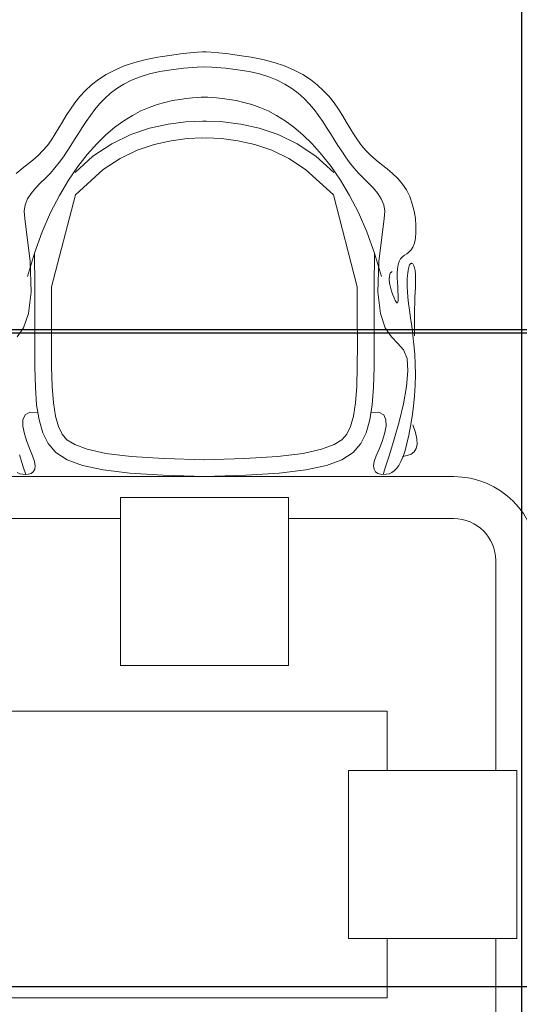
# Model space of a CAD drawing. Units: inches. Extents: x 1454 to 2136, y 626 to 1213.
# Tile 16 of 23: x 1678 to 1701, y 1095 to 1141. Entities that reach past the tile are written whole.
import ezdxf

# ---------------------------------------------------------------- set-up
doc = ezdxf.new("R2010")
doc.units = ezdxf.units.IN
doc.header["$MEASUREMENT"] = 0
for name, color, linetype, lineweight in [('A-ANNO-DIMS', 2, 'Continuous', 18), ('A-FURN-PATT', 252, 'Continuous', 13), ('conference', 41, 'Continuous', 18)]:
    doc.layers.add(name, color=color, linetype=linetype, lineweight=lineweight)
doc.styles.get("Standard").update_dxf_attribs({"font": 'arial.ttf'})
doc.dimstyles.get("Standard").update_dxf_attribs({"dimtxt": 4, "dimasz": 0.18, "dimexe": 0.18, "dimexo": 0.0625, "dimgap": 0.09, "dimtad": 0, "dimtih": 1, "dimtoh": 1, "dimdec": 0, "dimrnd": 6, "dimzin": 0, "dimdsep": 46, "dimlunit": 3, "dimtxsty": 'Standard', "dimcen": 0.09, "dimadec": 0, "dimazin": 0, "dimtfac": 1, "dimtdec": 0, "dimtofl": 0, "dimtmove": 0, "dimatfit": 3, "dimfxl": 1, "dimtolj": 1, "dimtzin": 0, "dimarcsym": 0})

# ---------------------------------------------------------------- blocks, each defined once
blk = doc.blocks.new('ОГ52_на12персон_стол2800х900')
for p, q in [((920.4, 772.5), (933.9, 776)), ((933.9, 776), (948, 778.8)), ((948, 778.8), (961.8, 780.9)), ((961.8, 780.9), (974.8, 782.6)), ((974.8, 782.6), (986.2, 783.7)), ((986.2, 783.7), (995.2, 784.5)), ((995.2, 784.5), (1001.2, 784.9)), ((1001.2, 784.9), (1003.4, 785)), ((1005.6, 784.9), (1003.4, 785)), ((1011.5, 784.5), (1005.6, 784.9)), ((1020.6, 783.7), (1011.5, 784.5)), ((1031.9, 782.6), (1020.6, 783.7)), ((1044.9, 780.9), (1031.9, 782.6)), ((1058.8, 778.8), (1044.9, 780.9)), ((1072.8, 776), (1058.8, 778.8)), ((1086.4, 772.5), (1072.8, 776)), ((886.5, 758), (896.6, 763.4)), ((896.6, 763.4), (907.9, 768.3)), ((907.9, 768.3), (920.4, 772.5)), ((950.1, 761.5), (963.6, 763.8)), ((963.6, 763.8), (978.4, 765.6)), ((978.4, 765.6), (994.8, 766.8)), ((994.8, 766.8), (1003.4, 767.1)), ((1012, 766.8), (1003.4, 767.1)), ((1028.3, 765.6), (1012, 766.8)), ((1043.1, 763.8), (1028.3, 765.6)), ((1056.7, 761.5), (1043.1, 763.8)), ((1098.8, 768.3), (1086.4, 772.5)), ((1110.1, 763.4), (1098.8, 768.3)), ((1120.3, 758), (1110.1, 763.4)), ((869, 745.6), (877.3, 752)), ((877.3, 752), (886.5, 758)), ((907.5, 746.6), (916.6, 751.2)), ((916.6, 751.2), (926.7, 755.2)), ((926.7, 755.2), (937.8, 758.7)), ((937.8, 758.7), (950.1, 761.5)), ((1068.9, 758.7), (1056.7, 761.5)), ((1080, 755.2), (1068.9, 758.7)), ((1090.1, 751.2), (1080, 755.2)), ((1099.2, 746.6), (1090.1, 751.2)), ((1129.5, 752), (1120.3, 758)), ((1137.7, 745.6), (1129.5, 752)), ((855, 731.7), (861.6, 738.8)), ((861.6, 738.8), (869, 745.6)), ((891.7, 735.7), (899.2, 741.4)), ((899.2, 741.4), (907.5, 746.6)), ((1107.5, 741.4), (1099.2, 746.6)), ((1115, 735.7), (1107.5, 741.4)), ((1145.1, 738.8), (1137.7, 745.6)), ((1151.7, 731.7), (1145.1, 738.8)), ((849.1, 724.4), (855, 731.7)), ((878.6, 723.1), (884.9, 729.6)), ((884.9, 729.6), (891.7, 735.7)), ((956.3, 724.9), (965.4, 727)), ((965.4, 727), (974.1, 728.5)), ((974.1, 728.5), (982, 729.6)), ((982, 729.6), (989.1, 730.4)), ((989.1, 730.4), (994.9, 730.8)), ((994.9, 730.8), (999.4, 731)), ((999.4, 731), (1002.3, 731.1)), ((1002.3, 731.1), (1003.4, 731.1)), ((1004.4, 731.1), (1003.4, 731.1)), ((1007.3, 731), (1004.4, 731.1)), ((1011.8, 730.8), (1007.3, 731)), ((1017.7, 730.4), (1011.8, 730.8)), ((1024.7, 729.6), (1017.7, 730.4)), ((1032.7, 728.5), (1024.7, 729.6)), ((1041.3, 727), (1032.7, 728.5)), ((1050.4, 724.9), (1041.3, 727)), ((1121.9, 729.6), (1115, 735.7)), ((1128.1, 723.1), (1121.9, 729.6)), ((1157.6, 724.4), (1151.7, 731.7)), ((839, 709.4), (843.8, 716.9)), ((843.8, 716.9), (849.1, 724.4)), ((867.6, 709.3), (872.9, 716.3)), ((872.9, 716.3), (878.6, 723.1)), ((927.6, 714.7), (937.4, 718.9)), ((937.4, 718.9), (947, 722.3)), ((947, 722.3), (956.3, 724.9)), ((1059.7, 722.3), (1050.4, 724.9)), ((1069.3, 718.9), (1059.7, 722.3)), ((1079.1, 714.7), (1069.3, 718.9)), ((1133.9, 716.3), (1128.1, 723.1)), ((1139.2, 709.3), (1133.9, 716.3)), ((1162.9, 716.9), (1157.6, 724.4)), ((1167.7, 709.4), (1162.9, 716.9)), ((834.5, 701.9), (839, 709.4)), ((862.6, 702.2), (867.6, 709.3)), ((907.4, 703), (917.6, 709.4)), ((917.6, 709.4), (927.6, 714.7)), ((1089.1, 709.4), (1079.1, 714.7)), ((1099.4, 703), (1089.1, 709.4)), ((1144.1, 702.2), (1139.2, 709.3)), ((1172.2, 701.9), (1167.7, 709.4)), ((825.8, 687.3), (830.2, 694.5)), ((830.2, 694.5), (834.5, 701.9)), ((853.4, 687.9), (857.9, 695)), ((857.9, 695), (862.6, 702.2)), ((886.2, 686.1), (896.9, 695.3)), ((896.9, 695.3), (907.4, 703)), ((915.6, 686.5), (938.1, 694.2)), ((938.1, 694.2), (960.2, 699)), ((960.2, 699), (981.3, 701.6)), ((981.3, 701.6), (1001, 702.5)), ((1001, 702.5), (1003.4, 702.4)), ((1005.7, 702.5), (1003.4, 702.4)), ((1025.4, 701.6), (1005.7, 702.5)), ((1046.5, 699), (1025.4, 701.6)), ((1068.6, 694.2), (1046.5, 699)), ((1091.2, 686.5), (1068.6, 694.2)), ((1109.9, 695.3), (1099.4, 703)), ((1120.6, 686.1), (1109.9, 695.3)), ((1148.8, 695), (1144.1, 702.2)), ((1153.4, 687.9), (1148.8, 695)), ((1176.6, 694.5), (1172.2, 701.9)), ((1180.9, 687.3), (1176.6, 694.5)), ((816.5, 673.7), (821.3, 680.3)), ((821.3, 680.3), (825.8, 687.3)), ((844.5, 673.7), (848.9, 680.7)), ((848.9, 680.7), (853.4, 687.9)), ((875.2, 675.4), (886.2, 686.1)), ((893, 675.6), (915.6, 686.5)), ((963.6, 679.3), (983, 681.7)), ((983, 681.7), (1001.3, 682.5)), ((1001.3, 682.5), (1003, 682.4)), ((1005.5, 682.5), (1003.8, 682.4)), ((1023.8, 681.7), (1005.5, 682.5)), ((1043.1, 679.3), (1023.8, 681.7)), ((1113.8, 675.6), (1091.2, 686.5)), ((1131.5, 675.4), (1120.6, 686.1)), ((1157.8, 680.7), (1153.4, 687.9)), ((1162.2, 673.7), (1157.8, 680.7)), ((1185.4, 680.3), (1180.9, 687.3)), ((1190.3, 673.7), (1185.4, 680.3)), ((811.2, 667.5), (816.5, 673.7)), ((840.1, 666.7), (844.5, 673.7)), ((864, 663), (875.2, 675.4)), ((870.7, 660.8), (893, 675.6)), ((923.2, 668), (943.5, 674.9)), ((943.5, 674.9), (963.6, 679.3)), ((1063.2, 674.9), (1043.1, 679.3)), ((1083.6, 668), (1063.2, 674.9)), ((1136, 660.8), (1113.8, 675.6)), ((1142.7, 663), (1131.5, 675.4)), ((1166.7, 666.7), (1162.2, 673.7)), ((1195.6, 667.5), (1190.3, 673.7)), ((799, 656.2), (805.3, 661.7)), ((805.3, 661.7), (811.2, 667.5)), ((830.6, 653.3), (835.5, 659.9)), ((835.5, 659.9), (840.1, 666.7)), ((849.4, 641.6), (870.7, 660.8)), ((852.8, 648.7), (864, 663)), ((883, 644.9), (902.9, 658.2)), ((902.9, 658.2), (923.2, 668)), ((1103.8, 658.2), (1083.6, 668)), ((1123.7, 644.9), (1103.8, 658.2)), ((1157.3, 641.6), (1136, 660.8)), ((1154, 648.7), (1142.7, 663)), ((1171.3, 659.9), (1166.7, 666.7)), ((1176.1, 653.3), (1171.3, 659.9)), ((1201.4, 661.7), (1195.6, 667.5)), ((1207.7, 656.2), (1201.4, 661.7)), ((779.5, 640.1), (785.9, 645.6)), ((785.9, 645.6), (792.5, 650.9)), ((792.5, 650.9), (799, 656.2)), ((820, 640.6), (825.5, 646.8)), ((825.5, 646.8), (830.6, 653.3)), ((841.6, 632.4), (852.8, 648.7)), ((849.8, 615), (883, 644.9)), ((1157, 615), (1123.7, 644.9)), ((1165.2, 632.4), (1154, 648.7)), ((1181.3, 646.8), (1176.1, 653.3)), ((1186.8, 640.6), (1181.3, 646.8)), ((1214.2, 650.9), (1207.7, 656.2)), ((1220.8, 645.6), (1214.2, 650.9)), ((1227.3, 640.1), (1220.8, 645.6)), ((808, 628.7), (814.1, 634.6)), ((814.1, 634.6), (820, 640.6)), ((1192.7, 634.6), (1186.8, 640.6)), ((1198.7, 628.7), (1192.7, 634.6)), ((1233.4, 634.2), (1227.3, 640.1)), ((1238.9, 627.7), (1233.4, 634.2)), ((797.1, 616.6), (802.3, 622.8)), ((802.3, 622.8), (808, 628.7)), ((830.7, 614.1), (841.6, 632.4)), ((1176.1, 614.1), (1165.2, 632.4)), ((1204.5, 622.8), (1198.7, 628.7)), ((1209.6, 616.6), (1204.5, 622.8)), ((1243.7, 620.6), (1238.9, 627.7)), ((790, 603), (792.9, 610.1)), ((792.9, 610.1), (797.1, 616.6)), ((820.1, 593.6), (830.7, 614.1)), ((849.8, 615), (821.5, 505.2)), ((1157, 615), (1185.3, 505.2)), ((1186.6, 593.6), (1176.1, 614.1)), ((1213.8, 610.1), (1209.6, 616.6)), ((1216.7, 603), (1213.8, 610.1)), ((1247.7, 612.7), (1243.7, 620.6)), ((1250.7, 604.2), (1247.7, 612.7)), ((788.8, 595.2), (790, 603)), ((1217.9, 595.2), (1216.7, 603)), ((1253, 595.4), (1250.7, 604.2)), ((789.6, 586.5), (788.8, 595.2)), ((789.6, 586.5), (796, 535.5)), ((810.2, 570.7), (820.1, 593.6)), ((1196.5, 570.7), (1186.6, 593.6)), ((1217.1, 586.5), (1210.8, 535.5)), ((1217.1, 586.5), (1217.9, 595.2)), ((1254.4, 586.6), (1253, 595.4)), ((1255.1, 578.1), (1254.4, 586.6)), ((1255.1, 570.2), (1255.1, 578.1)), ((801, 545.4), (810.2, 570.7)), ((1205.7, 545.4), (1196.5, 570.7)), ((1253.2, 557.2), (1254.5, 563.1)), ((1254.5, 563.1), (1255.1, 570.2)), ((1249.2, 549.3), (1251.4, 552.7)), ((1251.4, 552.7), (1253.2, 557.2)), ((792.7, 517.6), (801, 545.4)), ((801, 545.4), (801.5, 505.1)), ((1205.7, 545.4), (1205.3, 505.1)), ((1214, 517.6), (1205.7, 545.4)), ((1236.9, 538.5), (1239.1, 540.8)), ((1239.1, 540.8), (1241.5, 542.8)), ((1241.5, 542.8), (1244.1, 544.6)), ((1244.1, 544.6), (1246.7, 546.7)), ((1246.7, 546.7), (1249.2, 549.3)), ((796, 535.5), (797, 498.8)), ((1210.8, 535.5), (1209.7, 498.8)), ((1233.3, 526.8), (1234, 531.5)), ((1234, 531.5), (1235.2, 535.5)), ((1235.2, 535.5), (1236.9, 538.5)), ((1246.2, 527), (1246.6, 528.8)), ((1246.6, 528.8), (1247.1, 530.3)), ((1247.1, 530.3), (1247.6, 531.5)), ((1247.6, 531.5), (1248.1, 532.3)), ((1248.1, 532.3), (1248.7, 532.9)), ((1248.7, 532.9), (1249.2, 533.2)), ((1249.2, 533.2), (1249.7, 533.3)), ((1249.7, 533.3), (1250.2, 533.2)), ((1250.2, 533.2), (1250.7, 533)), ((1250.7, 533), (1251.2, 532.5)), ((1251.2, 532.5), (1251.6, 531.9)), ((1251.6, 531.9), (1252.1, 531.1)), ((1252.1, 531.1), (1252.5, 530.2)), ((1252.5, 530.2), (1252.9, 529.1)), ((1252.9, 529.1), (1253.3, 527.9)), ((1253.3, 527.9), (1253.6, 526.5)), ((1223.5, 518.2), (1223.3, 514.2)), ((1224.6, 521.4), (1223.5, 518.2)), ((1226.8, 523.4), (1224.6, 521.4)), ((1232.9, 521.5), (1233.3, 526.8)), ((1232.9, 516), (1232.9, 521.5)), ((1233.1, 510.3), (1232.9, 516)), ((1244.8, 514.9), (1245, 518.7)), ((1245, 518.7), (1245.3, 521.9)), ((1245.3, 521.9), (1245.7, 524.7)), ((1245.7, 524.7), (1246.2, 527)), ((1253.6, 526.5), (1254, 524.9)), ((1254, 524.9), (1254.2, 523.1)), ((1254.2, 523.1), (1254.5, 521)), ((1254.5, 521), (1254.6, 518.5)), ((1254.6, 518.5), (1254.7, 515.7)), ((801.5, 505.1), (801.5, 469.2)), ((821.5, 505.2), (821.5, 469.2)), ((1185.3, 505.2), (1185.3, 469.2)), ((1205.3, 505.1), (1205.3, 469.2)), ((1223.3, 514.2), (1223.7, 509.6)), ((1223.7, 509.6), (1224.7, 504.8)), ((1224.7, 504.8), (1226.1, 500.1)), ((1233.4, 504.9), (1233.1, 510.3)), ((1233.7, 499.8), (1233.4, 504.9)), ((1244.7, 510.5), (1244.8, 514.9)), ((1244.8, 505.4), (1244.7, 510.5)), ((1245.1, 499.6), (1244.8, 505.4)), ((1254.6, 508.5), (1254.5, 504)), ((1254.7, 512.3), (1254.6, 508.5)), ((1254.7, 515.7), (1254.7, 512.3)), ((797, 498.8), (794, 473.4)), ((1209.7, 498.8), (1212.8, 473.4)), ((1226.1, 500.1), (1227.6, 495.7)), ((1227.6, 495.7), (1229, 492)), ((1233.9, 495.4), (1233.7, 499.8)), ((1233.9, 491.8), (1233.9, 495.4)), ((1245.6, 493.1), (1245.1, 499.6)), ((1246.4, 485.6), (1245.6, 493.1)), ((1253.9, 493), (1253.7, 486.1)), ((1254.2, 498.9), (1253.9, 493)), ((1254.5, 504), (1254.2, 498.9)), ((1229, 492), (1230.3, 489.2)), ((1230.3, 489.2), (1231.4, 487.3)), ((1231.4, 487.3), (1232.3, 486.4)), ((1232.3, 486.4), (1233, 486.4)), ((1233, 486.4), (1233.5, 487.3)), ((1233.5, 487.3), (1233.8, 489.1)), ((1233.8, 489.1), (1233.9, 491.8)), ((1247.4, 477.3), (1246.4, 485.6)), ((1253.7, 486.1), (1253.4, 478.2)), ((794, 473.4), (788.1, 456.6)), ((801.5, 469.2), (801.4, 437.5)), ((821.5, 469.2), (821.4, 437.6)), ((1185.3, 469.2), (1185.4, 437.6)), ((1205.3, 469.2), (1205.4, 437.5)), ((1212.8, 473.4), (1218.6, 456.6)), ((1248.7, 468.2), (1247.4, 477.3)), ((1253.4, 478.2), (1253.3, 469.2)), ((1253.3, 469.2), (1253.3, 458.8)), ((1250, 458.3), (1248.7, 468.2)), ((1251.4, 447.8), (1250, 458.3)), ((1253.3, 458.8), (1253.4, 447.1)), ((788.1, 456.6), (780.7, 445.7)), ((1218.6, 456.6), (1226, 445.7)), ((1226, 445.7), (1233.6, 437.8)), ((1252.6, 436.7), (1251.4, 447.8)), ((801.4, 437.5), (801.5, 409.8)), ((821.4, 437.6), (821.5, 410.1)), ((1185.4, 437.6), (1185.3, 410.1)), ((1205.4, 437.5), (1205.3, 409.8)), ((1233.6, 437.8), (1240.2, 430.2)), ((1253.6, 425.1), (1252.6, 436.7)), ((1240.2, 430.2), (1244.5, 420)), ((1254.2, 413.1), (1253.6, 425.1)), ((1244.5, 420), (1245.6, 405.3)), ((1254.4, 400.7), (1254.2, 413.1)), ((801.5, 409.8), (802.2, 385.6)), ((821.5, 410.1), (822.1, 386.6)), ((1185.3, 410.1), (1184.6, 386.6)), ((1205.3, 409.8), (1204.6, 385.6)), ((1245.6, 405.3), (1243.9, 386.7)), ((1254.1, 388.2), (1254.4, 400.7)), ((1253.4, 375.5), (1254.1, 388.2)), ((802.2, 385.6), (803.7, 364.7)), ((822.1, 386.6), (823.6, 367)), ((1184.6, 386.6), (1183.1, 367)), ((1204.6, 385.6), (1203, 364.7)), ((1243.9, 386.7), (1240.1, 366)), ((1252.1, 363), (1253.4, 375.5)), ((803.7, 364.7), (806.5, 346.8)), ((823.6, 367), (826.1, 351.1)), ((1183.1, 367), (1180.6, 351.1)), ((1203, 364.7), (1200.2, 346.8)), ((1240.1, 366), (1235, 344.5)), ((787.3, 347.1), (789.9, 353)), ((789.9, 353), (795.6, 356.1)), ((795.6, 356.1), (805.1, 355.7)), ((1211.1, 356.1), (1201.6, 355.7)), ((1216.8, 353), (1211.1, 356.1)), ((1219.4, 347.1), (1216.8, 353)), ((1250.6, 350.9), (1252.1, 363)), ((787.3, 339.3), (787.3, 347.1)), ((806.5, 346.8), (810.9, 331.5)), ((826.1, 351.1), (829.6, 338.8)), ((1180.6, 351.1), (1177.1, 338.8)), ((1200.2, 346.8), (1195.9, 331.5)), ((1219.5, 339.3), (1219.4, 347.1)), ((1235, 344.5), (1229.2, 323.8)), ((1248.7, 339.4), (1250.6, 350.9)), ((1251.4, 341), (1254.7, 331.8)), ((789.1, 330.3), (787.3, 339.3)), ((792, 321), (789.1, 330.3)), ((810.9, 331.5), (817.3, 318.7)), ((829.6, 338.8), (834, 329.9)), ((834, 329.9), (839.8, 323.3)), ((1172.7, 329.9), (1166.9, 323.3)), ((1177.1, 338.8), (1172.7, 329.9)), ((1195.9, 331.5), (1189.5, 318.7)), ((1214.7, 321), (1217.7, 330.3)), ((1217.7, 330.3), (1219.5, 339.3)), ((1244.4, 318.9), (1246.6, 328.7)), ((1246.6, 328.7), (1248.7, 339.4)), ((1254.7, 331.8), (1256.3, 324.1)), ((795.5, 312), (792, 321)), ((817.3, 318.7), (826.6, 308)), ((839.8, 323.3), (849, 317.4)), ((849, 317.4), (863.9, 311.8)), ((1157.8, 317.4), (1142.8, 311.8)), ((1166.9, 323.3), (1157.8, 317.4)), ((1189.5, 318.7), (1180.2, 308)), ((1211.2, 312), (1214.7, 321)), ((1229.2, 323.8), (1223.6, 305.4)), ((1242.1, 310.4), (1244.4, 318.9)), ((1256.5, 317.8), (1255.3, 312.9)), ((1256.3, 324.1), (1256.5, 317.8)), ((783.1, 305.4), (787.8, 291)), ((798.9, 304.2), (795.5, 312)), ((826.6, 308), (839.9, 299.4)), ((863.9, 311.8), (886.1, 307)), ((886.1, 307), (916.3, 303.4)), ((1120.7, 307), (1090.5, 303.4)), ((1142.8, 311.8), (1120.7, 307)), ((1180.2, 308), (1166.8, 299.4)), ((1207.8, 304.2), (1211.2, 312)), ((1223.6, 305.4), (1218.9, 291)), ((1239.7, 303.2), (1242.1, 310.4)), ((1249.2, 306.2), (1244.6, 304.3)), ((1252.8, 309), (1249.2, 306.2)), ((1255.3, 312.9), (1252.8, 309)), ((798.9, 304.2), (801.3, 297.4)), ((801.3, 297.4), (802.1, 292.1)), ((839.9, 299.4), (858.3, 292.5)), ((916.3, 303.4), (955.2, 300.9)), ((955.2, 300.9), (1004, 299.3)), ((1051.5, 300.9), (1002.7, 299.3)), ((1090.5, 303.4), (1051.5, 300.9)), ((1166.8, 299.4), (1148.5, 292.5)), ((1205.4, 297.4), (1204.6, 292.1)), ((1207.8, 304.2), (1205.4, 297.4)), ((1234.7, 292.5), (1237.2, 297.3)), ((1237.2, 297.3), (1239.7, 303.2)), ((1244.6, 304.3), (1239.1, 303.1)), ((783.6, 282.8), (780.4, 284.1)), ((786.9, 282.1), (783.6, 282.8)), ((790.4, 281.8), (786.9, 282.1)), ((787.8, 291), (790.9, 281.9)), ((793.9, 282.2), (790.4, 281.8)), ((797.1, 283.2), (793.9, 282.2)), ((799.7, 285.1), (797.1, 283.2)), ((801.5, 288.1), (799.7, 285.1)), ((802.1, 292.1), (801.5, 288.1)), ((858.3, 292.5), (882.8, 287.3)), ((882.8, 287.3), (914.4, 283.5)), ((914.4, 283.5), (954.3, 280.9)), ((1092.3, 283.5), (1052.5, 280.9)), ((1124, 287.3), (1092.3, 283.5)), ((1148.5, 292.5), (1124, 287.3)), ((1204.6, 292.1), (1205.3, 288.1)), ((1205.3, 288.1), (1207, 285.1)), ((1207, 285.1), (1209.6, 283.2)), ((1209.6, 283.2), (1212.8, 282.2)), ((1212.8, 282.2), (1216.3, 281.8)), ((1218.9, 291), (1215.9, 281.9)), ((1216.3, 281.8), (1219.8, 282.1)), ((1219.8, 282.1), (1223.2, 282.8)), ((1223.2, 282.8), (1226.3, 284.1)), ((1226.3, 284.1), (1229.2, 286.1)), ((1229.2, 286.1), (1232, 288.8)), ((1232, 288.8), (1234.7, 292.5)), ((-1300, 279.3), (1300, 279.3)), ((954.3, 280.9), (1003.4, 279.3)), ((1052.5, 280.9), (1003.4, 279.3)), ((903.4, 254.3), (903.4, 54.3)), ((1103.4, 254.3), (903.4, 254.3)), ((1103.4, 54.3), (1103.4, 254.3)), ((603.4, 229.3), (903.4, 229.3)), ((1103.4, 229.3), (1300, 229.3)), ((1350, 179.3), (1350, -70.7)), ((903.4, 54.3), (1103.4, 54.3)), ((1220.7, 0), (-1220.7, 0)), ((1220.7, -70.7), (1220.7, 0)), ((1175, -270.7), (1175, -70.7)), ((1175, -70.7), (1375, -70.7)), ((1375, -70.7), (1375, -270.7)), ((1375, -270.7), (1175, -270.7)), ((1220.7, -341.4), (1220.7, -270.7)), ((1350, -270.7), (1350, -520.7)), ((-1220.7, -341.4), (1220.7, -341.4))]:
    blk.add_line(p, q)
for radius in [100, 50]:
    blk.add_arc((1300, 179.3), radius, 0, 90)
blk = doc.blocks.new('*D23')
at = {"layer": 'A-ANNO-DIMS', "color": 0, "lineweight": -2, "transparency": 16777216}
for p, q in [((1571.674, 1139.532), (1571.674, 1162.157)), ((1571.854, 1161.977), (1615.675, 1161.977)), ((1721.545, 1161.977), (1677.724, 1161.977)), ((1721.725, 1139.532), (1721.725, 1162.157))]:
    blk.add_line(p, q, dxfattribs=at)
at = {"layer": 'A-ANNO-DIMS', "color": 0, "transparency": 16777216}
for points in [[(1571.854, 1162.007), (1571.854, 1161.947), (1571.674, 1161.977)], [(1721.545, 1162.007), (1721.545, 1161.947), (1721.725, 1161.977)]]:
    blk.add_solid(points, dxfattribs=at)
at = {"layer": 'Defpoints', "color": 0, "transparency": 16777216}
for p in [(1721.725, 1161.977), (1571.674, 1139.469), (1721.725, 1139.469)]:
    blk.add_point(p, dxfattribs=at)
at = {"layer": 'A-ANNO-DIMS', "color": 0, "transparency": 16777216, "insert": (1646.7, 1161.977), "char_height": 4, "attachment_point": 5}
blk.add_mtext('\\A1;CONFERENCE SET 150', dxfattribs=at)
blk = doc.blocks.new('*D33')
at = {"layer": 'A-ANNO-DIMS', "color": 0, "lineweight": -2, "transparency": 16777216}
for p, q in [((2032.494, 1126.282), (1462.374, 1126.282)), ((1462.554, 1126.102), (1462.554, 1056.381)), ((1462.554, 982.462), (1462.554, 1052.184)), ((2032.494, 982.282), (1462.374, 982.282))]:
    blk.add_line(p, q, dxfattribs=at)
at = {"layer": 'A-ANNO-DIMS', "color": 0, "transparency": 16777216}
for points in [[(1462.524, 1126.102), (1462.584, 1126.102), (1462.554, 1126.282)], [(1462.524, 982.462), (1462.584, 982.462), (1462.554, 982.282)]]:
    blk.add_solid(points, dxfattribs=at)
at = {"layer": 'Defpoints', "color": 0, "transparency": 16777216}
for p in [(1462.554, 1126.282), (2032.556, 1126.282), (2032.556, 982.282)]:
    blk.add_point(p, dxfattribs=at)
at = {"layer": 'A-ANNO-DIMS', "color": 0, "transparency": 16777216, "insert": (1462.554, 1054.282), "char_height": 4, "attachment_point": 5}
blk.add_mtext('\\A1;144', dxfattribs=at)
blk = doc.blocks.new('*D45')
at = {"layer": 'A-ANNO-DIMS', "color": 0, "lineweight": -2, "transparency": 16777216}
for p, q in [((1654.556, 913.345), (1654.556, 1210.464)), ((1654.736, 1210.284), (1670.917, 1210.284)), ((1700.896, 1210.284), (1684.715, 1210.284)), ((1701.076, 909.11), (1701.076, 1210.464))]:
    blk.add_line(p, q, dxfattribs=at)
at = {"layer": 'A-ANNO-DIMS', "color": 0, "transparency": 16777216}
for points in [[(1654.736, 1210.314), (1654.736, 1210.254), (1654.556, 1210.284)], [(1700.896, 1210.314), (1700.896, 1210.254), (1701.076, 1210.284)]]:
    blk.add_solid(points, dxfattribs=at)
at = {"layer": 'Defpoints', "color": 0, "transparency": 16777216}
for p in [(1701.076, 1210.284), (1654.556, 913.282), (1701.076, 909.048)]:
    blk.add_point(p, dxfattribs=at)
at = {"layer": 'A-ANNO-DIMS', "color": 0, "transparency": 16777216, "insert": (1677.816, 1210.284), "char_height": 4, "attachment_point": 5}
blk.add_mtext('\\A1;46.52', dxfattribs=at)
blk = doc.blocks.new('*D54')
at = {"layer": 'A-ANNO-DIMS', "color": 0, "lineweight": -2, "transparency": 16777216}
for p, q in [((1879.494, 1126.282), (1462.374, 1126.282)), ((1462.554, 1126.102), (1462.554, 1078.915)), ((1462.554, 1027.462), (1462.554, 1074.65)), ((1879.494, 1027.282), (1462.374, 1027.282))]:
    blk.add_line(p, q, dxfattribs=at)
at = {"layer": 'A-ANNO-DIMS', "color": 0, "transparency": 16777216}
for points in [[(1462.524, 1126.102), (1462.584, 1126.102), (1462.554, 1126.282)], [(1462.524, 1027.462), (1462.584, 1027.462), (1462.554, 1027.282)]]:
    blk.add_solid(points, dxfattribs=at)
at = {"layer": 'Defpoints', "color": 0, "transparency": 16777216}
for p in [(1879.556, 1126.282), (1462.554, 1027.282), (1879.556, 1027.282)]:
    blk.add_point(p, dxfattribs=at)
at = {"layer": 'A-ANNO-DIMS', "color": 0, "transparency": 16777216, "insert": (1462.554, 1076.782), "char_height": 4, "attachment_point": 5}
blk.add_mtext('\\A1;99', dxfattribs=at)
blk = doc.blocks.new('*D68')
at = {"layer": 'A-ANNO-DIMS', "color": 0, "lineweight": -2, "transparency": 16777216}
for p, q in [((1659.724, 1027.329), (1659.724, 1210.464)), ((1659.904, 1210.284), (1675.092, 1210.284)), ((1704.128, 1210.284), (1688.939, 1210.284)), ((1704.308, 1027.329), (1704.308, 1210.464))]:
    blk.add_line(p, q, dxfattribs=at)
at = {"layer": 'A-ANNO-DIMS', "color": 0, "transparency": 16777216}
for points in [[(1659.904, 1210.314), (1659.904, 1210.254), (1659.724, 1210.284)], [(1704.128, 1210.314), (1704.128, 1210.254), (1704.308, 1210.284)]]:
    blk.add_solid(points, dxfattribs=at)
at = {"layer": 'Defpoints', "color": 0, "transparency": 16777216}
for p in [(1704.308, 1210.284), (1659.724, 1027.267), (1704.308, 1027.267)]:
    blk.add_point(p, dxfattribs=at)
at = {"layer": 'A-ANNO-DIMS', "color": 0, "transparency": 16777216, "insert": (1682.016, 1210.284), "char_height": 4, "attachment_point": 5}
blk.add_mtext('\\A1;44.58', dxfattribs=at)
blk = doc.blocks.new('*D73')
at = {"layer": 'A-ANNO-DIMS', "color": 0, "lineweight": -2, "transparency": 16777216}
for p, q in [((1985.096, 1126.439), (1462.374, 1126.439)), ((1462.554, 1126.259), (1462.554, 1113.178)), ((1462.554, 1095.83), (1462.554, 1108.911)), ((1966.644, 1095.65), (1462.374, 1095.65))]:
    blk.add_line(p, q, dxfattribs=at)
at = {"layer": 'A-ANNO-DIMS', "color": 0, "transparency": 16777216}
for points in [[(1462.524, 1126.259), (1462.584, 1126.259), (1462.554, 1126.439)], [(1462.524, 1095.83), (1462.584, 1095.83), (1462.554, 1095.65)]]:
    blk.add_solid(points, dxfattribs=at)
at = {"layer": 'Defpoints', "color": 0, "transparency": 16777216}
for p in [(1985.158, 1126.439), (1462.554, 1095.65), (1966.707, 1095.65)]:
    blk.add_point(p, dxfattribs=at)
at = {"layer": 'A-ANNO-DIMS', "color": 0, "transparency": 16777216, "insert": (1462.554, 1111.044), "char_height": 4, "attachment_point": 5}
blk.add_mtext('\\A1;30.79', dxfattribs=at)
blk = doc.blocks.new('*D76')
at = {"layer": 'A-ANNO-DIMS', "color": 0, "lineweight": -2, "transparency": 16777216}
for p, q in [((1962.644, 1095.65), (1462.374, 1095.65)), ((1462.554, 1095.47), (1462.554, 1073.782)), ((1462.554, 1047.83), (1462.554, 1069.517)), ((1914.644, 1047.65), (1462.374, 1047.65))]:
    blk.add_line(p, q, dxfattribs=at)
at = {"layer": 'A-ANNO-DIMS', "color": 0, "transparency": 16777216}
for points in [[(1462.524, 1095.47), (1462.584, 1095.47), (1462.554, 1095.65)], [(1462.524, 1047.83), (1462.584, 1047.83), (1462.554, 1047.65)]]:
    blk.add_solid(points, dxfattribs=at)
at = {"layer": 'Defpoints', "color": 0, "transparency": 16777216}
for p in [(1962.707, 1095.65), (1462.554, 1047.65), (1914.707, 1047.65)]:
    blk.add_point(p, dxfattribs=at)
at = {"layer": 'A-ANNO-DIMS', "color": 0, "transparency": 16777216, "insert": (1462.554, 1071.65), "char_height": 4, "attachment_point": 5}
blk.add_mtext('\\A1;48', dxfattribs=at)

msp = doc.modelspace()

# ---------------------------------------------------------------- hatches: boundary and pattern name
at = {"layer": 'A-FURN-PATT'}
h = msp.add_hatch(dxfattribs=at)
h.set_pattern_fill('ESCHER', color=256)
h.paths.add_polyline_path([(1511.3761, 923.7174, 1), (1525.379, 923.7174, 1)])
h.paths.add_polyline_path([(1525.379, 816.0542, 1), (1511.3761, 816.0542, 1)])
h.paths.add_polyline_path([(1525.379, 712.7345, 1), (1511.3761, 712.7345, 1)])
h.paths.add_polyline_path([(2070.5057, 794.3402, 1), (2056.5027, 794.3402, 1)])
h.paths.add_polyline_path([(2005.868, 1014.5578, 1), (1991.8651, 1014.5578, 1)])
h.paths.add_polyline_path([(1994.0647, 1066.7584, 1), (2008.0677, 1066.7584, 1)])
h.paths.add_polyline_path([(1919.5492, 1065.3848, 1), (1933.5521, 1065.3848, 1)])
h.paths.add_polyline_path([(1936.8517, 1013.7336, 1), (1922.8488, 1013.7336, 1)])
h.paths.add_polyline_path([(1824.6062, 1109.1557, 1), (1838.6091, 1109.1557, 1)])

# ---------------------------------------------------------------- block references
at = {"layer": 'conference', "xscale": 0.0393700787401575, "yscale": 0.0393700787401575, "zscale": 0.0393700787401575}
msp.add_blockref('ОГ52_на12персон_стол2800х900', (1646.6996, 1108.5647), dxfattribs=at)

# ---------------------------------------------------------------- dimensions: what is measured, and where the dimension line sits
at = {"layer": 'A-ANNO-DIMS'}
for base, p1, p2, picture, middle in [((1701.0763, 1210.2845), (1654.5563, 913.2825), (1701.0763, 909.0476), '*D45', (1677.8163, 1210.2845)), ((1704.308, 1210.2845), (1659.7237, 1027.2667), (1704.308, 1027.2667), '*D68', (1682.0158, 1210.2845))]:
    dim = msp.add_linear_dim(base=base, p1=p1, p2=p2, dimstyle='Standard', override={"dimdec": 2, "dimlfac": 1, "dimrnd": 0, "dimzin": 0, "dimdsep": 46, "dimlunit": 2}, dxfattribs=at)
    dim.commit()
    dim.dimension.update_dxf_attribs({"geometry": picture, "text_midpoint": middle})
dim = msp.add_linear_dim(base=(1721.7253, 1161.9768), p1=(1571.674, 1139.4691), p2=(1721.7253, 1139.4691), text='CONFERENCE SET <>', dimstyle='Standard', override={"dimdec": 0, "dimlfac": 1, "dimrnd": 0, "dimzin": 0, "dimdsep": 46, "dimlunit": 2}, dxfattribs=at)
dim.commit()
dim.dimension.update_dxf_attribs({"geometry": '*D23', "text_midpoint": (1646.6996, 1161.9768)})
for base, p1, p2, override, picture, middle in [((1462.5543, 1095.6495), (1985.1581, 1126.439), (1966.7068, 1095.6495), {"dimdec": 2, "dimlfac": 1, "dimrnd": 0, "dimzin": 0, "dimdsep": 46, "dimlunit": 2}, '*D73', (1462.5543, 1111.0443)), ((1462.5543, 1126.2825), (2032.5563, 982.2825), (2032.5563, 1126.2825), {"dimdec": 0, "dimlfac": 1, "dimrnd": 0, "dimzin": 0, "dimdsep": 46, "dimlunit": 2}, '*D33', (1462.5543, 1054.2825)), ((1462.5543, 1027.2825), (1879.5563, 1126.2825), (1879.5563, 1027.2825), {"dimdec": 0, "dimlfac": 1, "dimrnd": 0, "dimzin": 0, "dimdsep": 46, "dimlunit": 2}, '*D54', (1462.5543, 1076.7825)), ((1462.5543, 1047.6495), (1962.7068, 1095.6495), (1914.7068, 1047.6495), {"dimdec": 0, "dimlfac": 1, "dimrnd": 0, "dimzin": 0, "dimdsep": 46, "dimlunit": 2}, '*D76', (1462.5543, 1071.6495))]:
    dim = msp.add_linear_dim(base=base, p1=p1, p2=p2, angle=90, dimstyle='Standard', override=override, dxfattribs=at)
    dim.commit()
    dim.dimension.update_dxf_attribs({"geometry": picture, "text_midpoint": middle})

doc.saveas('drawing.dxf')
